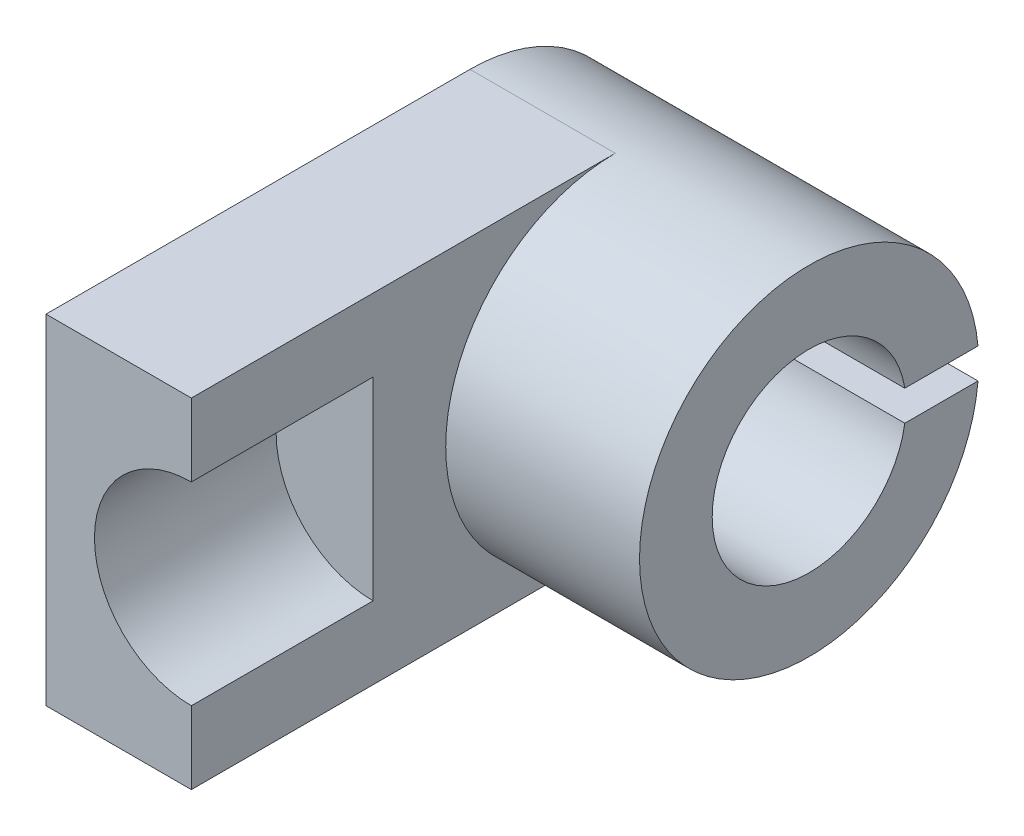
ISO-10303-21;
HEADER;
FILE_DESCRIPTION(('STEP AP214'),'2;1');
FILE_NAME('part.step','',(''),(''),'','','');
FILE_SCHEMA(('AUTOMOTIVE_DESIGN { 1 0 10303 214 1 1 1 1 }'));
ENDSEC;
DATA;
#1=APPLICATION_CONTEXT('core data for automotive mechanical design processes');
#2=APPLICATION_PROTOCOL_DEFINITION('international standard','automotive_design',2000,#1);
#3=PRODUCT_CONTEXT('',#1,'mechanical');
#4=PRODUCT('Part','Part','',(#3));
#5=PRODUCT_RELATED_PRODUCT_CATEGORY('part','',(#4));
#6=PRODUCT_DEFINITION_FORMATION('','',#4);
#7=PRODUCT_DEFINITION_CONTEXT('part definition',#1,'design');
#8=PRODUCT_DEFINITION('design','',#6,#7);
#9=PRODUCT_DEFINITION_SHAPE('','',#8);
#10=(LENGTH_UNIT() NAMED_UNIT(*) SI_UNIT(.MILLI.,.METRE.));
#11=(NAMED_UNIT(*) PLANE_ANGLE_UNIT() SI_UNIT($,.RADIAN.));
#12=(NAMED_UNIT(*) SI_UNIT($,.STERADIAN.) SOLID_ANGLE_UNIT());
#13=UNCERTAINTY_MEASURE_WITH_UNIT(LENGTH_MEASURE(1.E-05),#10,'distance_accuracy_value','');
#14=(GEOMETRIC_REPRESENTATION_CONTEXT(3) GLOBAL_UNCERTAINTY_ASSIGNED_CONTEXT((#13)) GLOBAL_UNIT_ASSIGNED_CONTEXT((#10,
#11,#12)) REPRESENTATION_CONTEXT('',''));
#15=CARTESIAN_POINT('',(0.,0.,0.));
#16=DIRECTION('',(0.,0.,1.));
#17=DIRECTION('',(1.,0.,0.));
#18=AXIS2_PLACEMENT_3D('',#15,#16,#17);
#19=CARTESIAN_POINT('',(56.,0.,0.));
#20=DIRECTION('',(-1.,0.,0.));
#21=DIRECTION('',(0.,0.,1.));
#22=AXIS2_PLACEMENT_3D('',#19,#20,#21);
#23=CYLINDRICAL_SURFACE('',#22,28.);
#24=CARTESIAN_POINT('',(0.,0.,0.));
#25=DIRECTION('',(1.,0.,0.));
#26=DIRECTION('',(0.,0.,-1.));
#27=AXIS2_PLACEMENT_3D('',#24,#25,#26);
#28=CIRCLE('',#27,28.);
#29=CARTESIAN_POINT('',(0.,-28.,0.));
#30=VERTEX_POINT('',#29);
#31=CARTESIAN_POINT('',(0.,-2.5,-27.8881695347687));
#32=VERTEX_POINT('',#31);
#33=EDGE_CURVE('E132',#30,#32,#28,.T.);
#34=ORIENTED_EDGE('',*,*,#33,.T.);
#35=DIRECTION('',(-1.,0.,0.));
#36=VECTOR('',#35,1.);
#37=CARTESIAN_POINT('',(56.,-2.5,-27.8881695347687));
#38=LINE('',#37,#36);
#39=CARTESIAN_POINT('',(56.,-2.5,-27.8881695347687));
#40=VERTEX_POINT('',#39);
#41=EDGE_CURVE('E153',#32,#40,#38,.F.);
#42=ORIENTED_EDGE('',*,*,#41,.T.);
#43=CARTESIAN_POINT('',(56.,0.,0.));
#44=DIRECTION('',(1.,0.,0.));
#45=DIRECTION('',(0.,0.,-1.));
#46=AXIS2_PLACEMENT_3D('',#43,#44,#45);
#47=CIRCLE('',#46,28.);
#48=CARTESIAN_POINT('',(56.,2.5,-27.8881695347687));
#49=VERTEX_POINT('',#48);
#50=EDGE_CURVE('E123',#49,#40,#47,.T.);
#51=ORIENTED_EDGE('',*,*,#50,.F.);
#52=DIRECTION('',(-1.,0.,0.));
#53=VECTOR('',#52,1.);
#54=CARTESIAN_POINT('',(56.,2.5,-27.8881695347687));
#55=LINE('',#54,#53);
#56=CARTESIAN_POINT('',(0.,2.5,-27.8881695347687));
#57=VERTEX_POINT('',#56);
#58=EDGE_CURVE('E150',#49,#57,#55,.T.);
#59=ORIENTED_EDGE('',*,*,#58,.T.);
#60=CARTESIAN_POINT('',(0.,28.,0.));
#61=VERTEX_POINT('',#60);
#62=EDGE_CURVE('E129',#57,#61,#28,.T.);
#63=ORIENTED_EDGE('',*,*,#62,.T.);
#64=DIRECTION('',(-1.,0.,0.));
#65=VECTOR('',#64,1.);
#66=CARTESIAN_POINT('',(24.,28.,0.));
#67=LINE('',#66,#65);
#68=CARTESIAN_POINT('',(24.,28.,0.));
#69=VERTEX_POINT('',#68);
#70=EDGE_CURVE('E186',#69,#61,#67,.T.);
#71=ORIENTED_EDGE('',*,*,#70,.F.);
#72=CARTESIAN_POINT('',(24.,0.,0.));
#73=DIRECTION('',(1.,0.,0.));
#74=DIRECTION('',(0.,0.,-1.));
#75=AXIS2_PLACEMENT_3D('',#72,#73,#74);
#76=CIRCLE('',#75,28.);
#77=CARTESIAN_POINT('',(24.,-28.,0.));
#78=VERTEX_POINT('',#77);
#79=EDGE_CURVE('E133',#69,#78,#76,.T.);
#80=ORIENTED_EDGE('',*,*,#79,.T.);
#81=DIRECTION('',(-1.,0.,0.));
#82=VECTOR('',#81,1.);
#83=CARTESIAN_POINT('',(24.,-28.,0.));
#84=LINE('',#83,#82);
#85=EDGE_CURVE('E176',#78,#30,#84,.T.);
#86=ORIENTED_EDGE('',*,*,#85,.T.);
#87=EDGE_LOOP('',(#34,#42,#51,#59,#63,#71,#80,#86));
#88=FACE_BOUND('',#87,.T.);
#89=ADVANCED_FACE('F39',(#88),#23,.T.);
#90=CARTESIAN_POINT('',(56.,0.,0.));
#91=DIRECTION('',(1.,0.,0.));
#92=DIRECTION('',(0.,0.,-1.));
#93=AXIS2_PLACEMENT_3D('',#90,#91,#92);
#94=PLANE('',#93);
#95=DIRECTION('',(0.,0.,-1.));
#96=VECTOR('',#95,1.);
#97=CARTESIAN_POINT('',(56.,-2.5,0.));
#98=LINE('',#97,#96);
#99=CARTESIAN_POINT('',(56.,-2.49999999999999,-15.8034806292791));
#100=VERTEX_POINT('',#99);
#101=EDGE_CURVE('E114',#100,#40,#98,.T.);
#102=ORIENTED_EDGE('',*,*,#101,.F.);
#103=CARTESIAN_POINT('',(56.,0.,0.));
#104=DIRECTION('',(1.,0.,0.));
#105=DIRECTION('',(0.,0.,-1.));
#106=AXIS2_PLACEMENT_3D('',#103,#104,#105);
#107=CIRCLE('',#106,16.);
#108=CARTESIAN_POINT('',(56.,2.5,-15.8034806292791));
#109=VERTEX_POINT('',#108);
#110=EDGE_CURVE('E124',#109,#100,#107,.T.);
#111=ORIENTED_EDGE('',*,*,#110,.F.);
#112=DIRECTION('',(0.,0.,1.));
#113=VECTOR('',#112,1.);
#114=CARTESIAN_POINT('',(56.,2.5,0.));
#115=LINE('',#114,#113);
#116=EDGE_CURVE('E52',#49,#109,#115,.T.);
#117=ORIENTED_EDGE('',*,*,#116,.F.);
#118=ORIENTED_EDGE('',*,*,#50,.T.);
#119=EDGE_LOOP('',(#102,#111,#117,#118));
#120=FACE_BOUND('',#119,.T.);
#121=ADVANCED_FACE('F125',(#120),#94,.T.);
#122=CARTESIAN_POINT('',(0.,0.,0.));
#123=DIRECTION('',(1.,0.,0.));
#124=DIRECTION('',(0.,0.,-1.));
#125=AXIS2_PLACEMENT_3D('',#122,#123,#124);
#126=PLANE('',#125);
#127=CARTESIAN_POINT('',(0.,0.,0.));
#128=DIRECTION('',(1.,0.,0.));
#129=DIRECTION('',(0.,0.,-1.));
#130=AXIS2_PLACEMENT_3D('',#127,#128,#129);
#131=CIRCLE('',#130,16.);
#132=CARTESIAN_POINT('',(0.,2.5,-15.8034806292791));
#133=VERTEX_POINT('',#132);
#134=CARTESIAN_POINT('',(0.,-2.5,-15.8034806292791));
#135=VERTEX_POINT('',#134);
#136=EDGE_CURVE('E128',#133,#135,#131,.T.);
#137=ORIENTED_EDGE('',*,*,#136,.T.);
#138=DIRECTION('',(0.,0.,-1.));
#139=VECTOR('',#138,1.);
#140=CARTESIAN_POINT('',(0.,-2.5,0.));
#141=LINE('',#140,#139);
#142=EDGE_CURVE('E58',#135,#32,#141,.T.);
#143=ORIENTED_EDGE('',*,*,#142,.T.);
#144=ORIENTED_EDGE('',*,*,#33,.F.);
#145=DIRECTION('',(0.,0.,1.));
#146=VECTOR('',#145,1.);
#147=CARTESIAN_POINT('',(0.,-28.,70.));
#148=LINE('',#147,#146);
#149=CARTESIAN_POINT('',(0.,-28.,70.));
#150=VERTEX_POINT('',#149);
#151=EDGE_CURVE('E164',#30,#150,#148,.T.);
#152=ORIENTED_EDGE('',*,*,#151,.T.);
#153=DIRECTION('',(0.,1.,0.));
#154=VECTOR('',#153,1.);
#155=CARTESIAN_POINT('',(0.,28.,70.));
#156=LINE('',#155,#154);
#157=CARTESIAN_POINT('',(0.,28.,70.));
#158=VERTEX_POINT('',#157);
#159=EDGE_CURVE('E185',#150,#158,#156,.T.);
#160=ORIENTED_EDGE('',*,*,#159,.T.);
#161=DIRECTION('',(0.,0.,-1.));
#162=VECTOR('',#161,1.);
#163=CARTESIAN_POINT('',(0.,28.,0.));
#164=LINE('',#163,#162);
#165=EDGE_CURVE('E172',#158,#61,#164,.T.);
#166=ORIENTED_EDGE('',*,*,#165,.T.);
#167=ORIENTED_EDGE('',*,*,#62,.F.);
#168=DIRECTION('',(0.,0.,1.));
#169=VECTOR('',#168,1.);
#170=CARTESIAN_POINT('',(0.,2.5,0.));
#171=LINE('',#170,#169);
#172=EDGE_CURVE('E127',#57,#133,#171,.T.);
#173=ORIENTED_EDGE('',*,*,#172,.T.);
#174=EDGE_LOOP('',(#137,#143,#144,#152,#160,#166,#167,#173));
#175=FACE_BOUND('',#174,.T.);
#176=ADVANCED_FACE('F144',(#175),#126,.F.);
#177=CARTESIAN_POINT('',(56.,0.,0.));
#178=DIRECTION('',(-1.,0.,0.));
#179=DIRECTION('',(0.,0.,1.));
#180=AXIS2_PLACEMENT_3D('',#177,#178,#179);
#181=CYLINDRICAL_SURFACE('',#180,16.);
#182=DIRECTION('',(-1.,0.,0.));
#183=VECTOR('',#182,1.);
#184=CARTESIAN_POINT('',(56.,-2.5,-15.8034806292791));
#185=LINE('',#184,#183);
#186=EDGE_CURVE('E11',#135,#100,#185,.F.);
#187=ORIENTED_EDGE('',*,*,#186,.F.);
#188=ORIENTED_EDGE('',*,*,#136,.F.);
#189=DIRECTION('',(-1.,0.,0.));
#190=VECTOR('',#189,1.);
#191=CARTESIAN_POINT('',(56.,2.5,-15.8034806292791));
#192=LINE('',#191,#190);
#193=EDGE_CURVE('E46',#109,#133,#192,.T.);
#194=ORIENTED_EDGE('',*,*,#193,.F.);
#195=ORIENTED_EDGE('',*,*,#110,.T.);
#196=EDGE_LOOP('',(#187,#188,#194,#195));
#197=FACE_BOUND('',#196,.T.);
#198=ADVANCED_FACE('F126',(#197),#181,.F.);
#199=CARTESIAN_POINT('',(24.,28.,0.));
#200=DIRECTION('',(0.,1.,0.));
#201=DIRECTION('',(0.,0.,1.));
#202=AXIS2_PLACEMENT_3D('',#199,#200,#201);
#203=PLANE('',#202);
#204=ORIENTED_EDGE('',*,*,#165,.F.);
#205=DIRECTION('',(-1.,0.,0.));
#206=VECTOR('',#205,1.);
#207=CARTESIAN_POINT('',(24.,28.,70.));
#208=LINE('',#207,#206);
#209=CARTESIAN_POINT('',(24.,28.,70.));
#210=VERTEX_POINT('',#209);
#211=EDGE_CURVE('E188',#210,#158,#208,.T.);
#212=ORIENTED_EDGE('',*,*,#211,.F.);
#213=DIRECTION('',(0.,0.,-1.));
#214=VECTOR('',#213,1.);
#215=CARTESIAN_POINT('',(24.,28.,0.));
#216=LINE('',#215,#214);
#217=EDGE_CURVE('E177',#210,#69,#216,.T.);
#218=ORIENTED_EDGE('',*,*,#217,.T.);
#219=ORIENTED_EDGE('',*,*,#70,.T.);
#220=EDGE_LOOP('',(#204,#212,#218,#219));
#221=FACE_BOUND('',#220,.T.);
#222=ADVANCED_FACE('F209',(#221),#203,.T.);
#223=CARTESIAN_POINT('',(24.,28.,70.));
#224=DIRECTION('',(0.,0.,1.));
#225=DIRECTION('',(1.,0.,0.));
#226=AXIS2_PLACEMENT_3D('',#223,#224,#225);
#227=PLANE('',#226);
#228=CARTESIAN_POINT('',(24.,0.,70.));
#229=DIRECTION('',(0.,0.,1.));
#230=DIRECTION('',(1.,0.,0.));
#231=AXIS2_PLACEMENT_3D('',#228,#229,#230);
#232=CIRCLE('',#231,16.);
#233=CARTESIAN_POINT('',(24.,16.,70.));
#234=VERTEX_POINT('',#233);
#235=CARTESIAN_POINT('',(24.,-16.,70.));
#236=VERTEX_POINT('',#235);
#237=EDGE_CURVE('E154',#234,#236,#232,.T.);
#238=ORIENTED_EDGE('',*,*,#237,.F.);
#239=DIRECTION('',(0.,1.,0.));
#240=VECTOR('',#239,1.);
#241=CARTESIAN_POINT('',(24.,28.,70.));
#242=LINE('',#241,#240);
#243=EDGE_CURVE('E171',#234,#210,#242,.T.);
#244=ORIENTED_EDGE('',*,*,#243,.T.);
#245=ORIENTED_EDGE('',*,*,#211,.T.);
#246=ORIENTED_EDGE('',*,*,#159,.F.);
#247=DIRECTION('',(-1.,0.,0.));
#248=VECTOR('',#247,1.);
#249=CARTESIAN_POINT('',(24.,-28.,70.));
#250=LINE('',#249,#248);
#251=CARTESIAN_POINT('',(24.,-28.,70.));
#252=VERTEX_POINT('',#251);
#253=EDGE_CURVE('E192',#252,#150,#250,.T.);
#254=ORIENTED_EDGE('',*,*,#253,.F.);
#255=EDGE_CURVE('E174',#252,#236,#242,.T.);
#256=ORIENTED_EDGE('',*,*,#255,.T.);
#257=EDGE_LOOP('',(#238,#244,#245,#246,#254,#256));
#258=FACE_BOUND('',#257,.T.);
#259=ADVANCED_FACE('F204',(#258),#227,.T.);
#260=CARTESIAN_POINT('',(24.,-28.,70.));
#261=DIRECTION('',(0.,-1.,0.));
#262=DIRECTION('',(0.,0.,-1.));
#263=AXIS2_PLACEMENT_3D('',#260,#261,#262);
#264=PLANE('',#263);
#265=ORIENTED_EDGE('',*,*,#151,.F.);
#266=ORIENTED_EDGE('',*,*,#85,.F.);
#267=DIRECTION('',(0.,0.,1.));
#268=VECTOR('',#267,1.);
#269=CARTESIAN_POINT('',(24.,-28.,70.));
#270=LINE('',#269,#268);
#271=EDGE_CURVE('E169',#78,#252,#270,.T.);
#272=ORIENTED_EDGE('',*,*,#271,.T.);
#273=ORIENTED_EDGE('',*,*,#253,.T.);
#274=EDGE_LOOP('',(#265,#266,#272,#273));
#275=FACE_BOUND('',#274,.T.);
#276=ADVANCED_FACE('F200',(#275),#264,.T.);
#277=CARTESIAN_POINT('',(24.,0.,0.));
#278=DIRECTION('',(1.,0.,0.));
#279=DIRECTION('',(0.,0.,-1.));
#280=AXIS2_PLACEMENT_3D('',#277,#278,#279);
#281=PLANE('',#280);
#282=DIRECTION('',(0.,0.,1.));
#283=VECTOR('',#282,1.);
#284=CARTESIAN_POINT('',(24.,16.,40.));
#285=LINE('',#284,#283);
#286=CARTESIAN_POINT('',(24.,16.,40.));
#287=VERTEX_POINT('',#286);
#288=EDGE_CURVE('E162',#287,#234,#285,.T.);
#289=ORIENTED_EDGE('',*,*,#288,.F.);
#290=DIRECTION('',(0.,1.,0.));
#291=VECTOR('',#290,1.);
#292=CARTESIAN_POINT('',(24.,16.,40.));
#293=LINE('',#292,#291);
#294=CARTESIAN_POINT('',(24.,-16.,40.));
#295=VERTEX_POINT('',#294);
#296=EDGE_CURVE('E158',#295,#287,#293,.T.);
#297=ORIENTED_EDGE('',*,*,#296,.F.);
#298=DIRECTION('',(0.,0.,1.));
#299=VECTOR('',#298,1.);
#300=CARTESIAN_POINT('',(24.,-16.,40.));
#301=LINE('',#300,#299);
#302=EDGE_CURVE('E161',#295,#236,#301,.T.);
#303=ORIENTED_EDGE('',*,*,#302,.T.);
#304=ORIENTED_EDGE('',*,*,#255,.F.);
#305=ORIENTED_EDGE('',*,*,#271,.F.);
#306=ORIENTED_EDGE('',*,*,#79,.F.);
#307=ORIENTED_EDGE('',*,*,#217,.F.);
#308=ORIENTED_EDGE('',*,*,#243,.F.);
#309=EDGE_LOOP('',(#289,#297,#303,#304,#305,#306,#307,#308));
#310=FACE_BOUND('',#309,.T.);
#311=ADVANCED_FACE('F213',(#310),#281,.T.);
#312=CARTESIAN_POINT('',(24.,0.,40.));
#313=DIRECTION('',(0.,0.,1.));
#314=DIRECTION('',(1.,0.,0.));
#315=AXIS2_PLACEMENT_3D('',#312,#313,#314);
#316=CYLINDRICAL_SURFACE('',#315,16.);
#317=ORIENTED_EDGE('',*,*,#237,.T.);
#318=ORIENTED_EDGE('',*,*,#302,.F.);
#319=CARTESIAN_POINT('',(24.,0.,40.));
#320=DIRECTION('',(0.,0.,1.));
#321=DIRECTION('',(1.,0.,0.));
#322=AXIS2_PLACEMENT_3D('',#319,#320,#321);
#323=CIRCLE('',#322,16.);
#324=EDGE_CURVE('E156',#287,#295,#323,.T.);
#325=ORIENTED_EDGE('',*,*,#324,.F.);
#326=ORIENTED_EDGE('',*,*,#288,.T.);
#327=EDGE_LOOP('',(#317,#318,#325,#326));
#328=FACE_BOUND('',#327,.T.);
#329=ADVANCED_FACE('F220',(#328),#316,.F.);
#330=CARTESIAN_POINT('',(24.,0.,40.));
#331=DIRECTION('',(0.,0.,1.));
#332=DIRECTION('',(1.,0.,0.));
#333=AXIS2_PLACEMENT_3D('',#330,#331,#332);
#334=PLANE('',#333);
#335=ORIENTED_EDGE('',*,*,#324,.T.);
#336=ORIENTED_EDGE('',*,*,#296,.T.);
#337=EDGE_LOOP('',(#335,#336));
#338=FACE_BOUND('',#337,.T.);
#339=ADVANCED_FACE('F218',(#338),#334,.T.);
#340=CARTESIAN_POINT('',(-24.,2.5,0.));
#341=DIRECTION('',(0.,1.,0.));
#342=DIRECTION('',(0.,0.,1.));
#343=AXIS2_PLACEMENT_3D('',#340,#341,#342);
#344=PLANE('',#343);
#345=ORIENTED_EDGE('',*,*,#116,.T.);
#346=ORIENTED_EDGE('',*,*,#193,.T.);
#347=ORIENTED_EDGE('',*,*,#172,.F.);
#348=ORIENTED_EDGE('',*,*,#58,.F.);
#349=EDGE_LOOP('',(#345,#346,#347,#348));
#350=FACE_BOUND('',#349,.T.);
#351=ADVANCED_FACE('F143',(#350),#344,.F.);
#352=CARTESIAN_POINT('',(-24.,-2.5,0.));
#353=DIRECTION('',(0.,-1.,0.));
#354=DIRECTION('',(0.,0.,-1.));
#355=AXIS2_PLACEMENT_3D('',#352,#353,#354);
#356=PLANE('',#355);
#357=ORIENTED_EDGE('',*,*,#142,.F.);
#358=ORIENTED_EDGE('',*,*,#186,.T.);
#359=ORIENTED_EDGE('',*,*,#101,.T.);
#360=ORIENTED_EDGE('',*,*,#41,.F.);
#361=EDGE_LOOP('',(#357,#358,#359,#360));
#362=FACE_BOUND('',#361,.T.);
#363=ADVANCED_FACE('F115',(#362),#356,.F.);
#364=CLOSED_SHELL('',(#89,#121,#176,#198,#222,#259,#276,#311,#329,#339,#351,#363));
#365=MANIFOLD_SOLID_BREP('B2',#364);
#366=ADVANCED_BREP_SHAPE_REPRESENTATION('',(#18,#365),#14);
#367=SHAPE_DEFINITION_REPRESENTATION(#9,#366);
ENDSEC;
END-ISO-10303-21;
